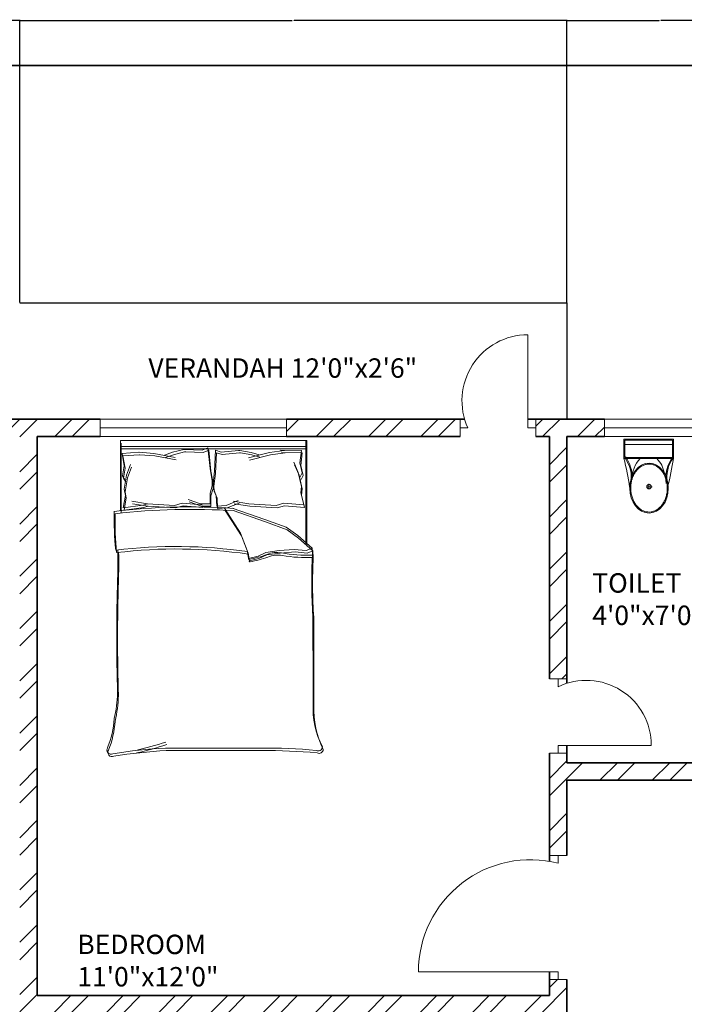
# Model space of a CAD drawing. Units: inches. Extents: x 1885 to 2748, y 783 to 2421.
# Tile 89 of 117: x 2170 to 2341, y 2167 to 2421. Entities that reach past the tile are written whole.
import ezdxf

# ---------------------------------------------------------------- set-up
doc = ezdxf.new("R2010")
doc.units = ezdxf.units.IN
for name, color, linetype, lineweight in [('A-ANNO-DIMS', 2, 'Continuous', 18), ('A-ANNO-TTLB', 7, 'Continuous', 35), ('A-AREA-IDEN', 7, 'Continuous', 18), ('A-DOOR', 31, 'Continuous', 18), ('A-FLOR-BALC', 7, 'Continuous', 25), ('A-FLOR-FIXT', 8, 'Continuous', 18), ('A-FURN', 8, 'Continuous', 13), ('A-GLAZ', 181, 'Continuous', 18), ('A-WALL', 7, 'Continuous', 35)]:
    doc.layers.add(name, color=color, linetype=linetype, lineweight=lineweight)
doc.layers.add('A-WALL-PATT', color=85, linetype='Continuous', lineweight=13, true_color=0x58ba48)
doc.styles.get("Standard").update_dxf_attribs({"font": 'arial.ttf'})
doc.dimstyles.get("Standard").update_dxf_attribs({"dimtxt": 0.18, "dimasz": 0.18, "dimexe": 0.18, "dimexo": 0.0625, "dimgap": 0.09, "dimtad": 0, "dimtih": 1, "dimtoh": 1, "dimdec": 4, "dimzin": 0, "dimdsep": 46, "dimtxsty": 'Standard', "dimcen": 0.09, "dimadec": 0, "dimazin": 0, "dimtfac": 1, "dimtdec": 4, "dimtofl": 0, "dimtmove": 0, "dimatfit": 3, "dimfxl": 1, "dimtolj": 1, "dimtzin": 0, "dimarcsym": 0})

# ---------------------------------------------------------------- blocks, each defined once
blk = doc.blocks.new('A$C31115884')
for p, q in [((258, 466), (258, 523)), ((283, 498), (223, 498)), ((0, 200), (0, 0)), ((520, 200), (0, 200)), ((10, 190), (10, 10)), ((510, 190), (10, 190)), ((510, 10), (510, 190)), ((520, 0), (520, 200)), ((510, 54), (0, 54)), ((10, 10), (510, 10)), ((0, 0), (520, 0))]:
    blk.add_line(p, q)
blk.add_circle((256, 496), 23.6)
for centre, radius, start, end in [((2778, -205), 2807, 165.4549, 171.7133), ((-295, 403), 365, 324.2091, 9.3499), ((-295, 403), 375, 324.2091, 9.3499), ((139, 406), 293, 315.8436, 2.6563), ((806, 403), 365, 170.6501, 215.7909), ((3237, 905), 2807, 188.2867, 194.5451), ((384, 406), 293, 190.2774, 224.1564), ((806, 403), 375, 179.2036, 215.7909)]:
    blk.add_arc(centre, radius, start, end)
blk.add_ellipse((256, 510), major_axis=(0, -261), ratio=0.772727)
blk.add_open_spline([(256, 259), (263, 259), (270, 260), (288, 262), (299, 265), (320, 273), (330, 278), (350, 291), (360, 299), (378, 316), (386, 326), (402, 347), (409, 358), (421, 383), (427, 395), (436, 422), (440, 436), (445, 465), (447, 480), (448, 509), (448, 524), (445, 553), (443, 568), (436, 596), (432, 610), (422, 636), (416, 649), (402, 672), (395, 683), (379, 703), (370, 712), (351, 728), (341, 735), (321, 746), (310, 751), (289, 757), (278, 759), (256, 761), (245, 761), (223, 757), (212, 754), (191, 746), (181, 741), (161, 728), (151, 720), (133, 703), (125, 693), (110, 672), (103, 660), (90, 636), (85, 623), (76, 596), (72, 582), (67, 553), (66, 538), (64, 509), (65, 494), (68, 465), (70, 450), (77, 422), (81, 408), (91, 382), (97, 370), (111, 346), (118, 335), (135, 316), (144, 307), (162, 291), (172, 284), (193, 273), (203, 269), (225, 262), (236, 260), (250, 259), (253, 259), (256, 259)], degree=3, knots=[0, 0, 0, 0, 0.110105, 0.110105, 0.285049, 0.285049, 0.459994, 0.459994, 0.634938, 0.634938, 0.809882, 0.809882, 0.984827, 0.984827, 1.159771, 1.159771, 1.334715, 1.334715, 1.50966, 1.50966, 1.684604, 1.684604, 1.859549, 1.859549, 2.034493, 2.034493, 2.209437, 2.209437, 2.384382, 2.384382, 2.559326, 2.559326, 2.73427, 2.73427, 2.909215, 2.909215, 3.084159, 3.084159, 3.259103, 3.259103, 3.434048, 3.434048, 3.608992, 3.608992, 3.783936, 3.783936, 3.958881, 3.958881, 4.133825, 4.133825, 4.30877, 4.30877, 4.483714, 4.483714, 4.658658, 4.658658, 4.833603, 4.833603, 5.008547, 5.008547, 5.183491, 5.183491, 5.358436, 5.358436, 5.53338, 5.53338, 5.708324, 5.708324, 5.883269, 5.883269, 6.058213, 6.058213, 6.233158, 6.233158, 6.283185, 6.283185, 6.283185, 6.283185])
blk = doc.blocks.new('BED-DOUBLE')
for p, q in [((0, 51.49), (0.64, 51.49)), ((0, 3.47), (0, 51.49)), ((0, 51.26), (26.61, 51.26)), ((0, 51.26), (26.61, 51.26)), ((0.64, 51.49), (27.25, 51.49)), ((0.64, 51.49), (27.25, 51.49)), ((1.54, 3.47), (1.54, 51.26)), ((1.54, 3.47), (1.54, 51.26)), ((2.18, 3.7), (2.18, 51.49)), ((2.18, 3.7), (2.18, 51.49)), ((17.22, 50.93), (14.08, 50.15)), ((17.22, 50.93), (14.08, 50.15)), ((16.81, 45.79), (17.22, 50.93)), ((16.81, 45.79), (17.22, 50.93)), ((27.75, 52.87), (24.5, 49.16)), ((27.75, 52.87), (24.5, 49.16)), ((28.39, 53.09), (25.14, 49.39)), ((28.39, 53.09), (25.14, 49.39)), ((29.49, 52.95), (27.75, 52.87, 3.87)), ((29.49, 52.95), (27.75, 52.87, 3.87)), ((28.37, 51.33), (27.75, 52.87)), ((28.37, 51.33), (27.75, 52.87)), ((28.06, 48.23), (28.37, 51.33)), ((28.06, 48.23), (28.37, 51.33)), ((30.13, 53.17), (28.39, 53.09, 3.87)), ((30.13, 53.17), (28.39, 53.09, 3.87)), ((29.01, 51.56), (28.39, 53.09)), ((29.01, 51.56), (28.39, 53.09)), ((28.7, 48.46), (29.01, 51.56)), ((28.7, 48.46), (29.01, 51.56)), ((2.56, 50.11), (2.46, 44.71)), ((2.56, 50.11), (2.46, 44.71)), ((2.56, 50.11), (5.77, 49.73)), ((2.56, 50.11), (5.77, 49.73)), ((3.2, 50.34), (3.1, 44.94)), ((3.2, 50.34), (3.1, 44.94)), ((3.2, 50.34), (6.41, 49.96)), ((3.2, 50.34), (6.41, 49.96)), ((8.26, 49.31), (5.58, 48.13)), ((8.26, 49.31), (5.58, 48.13)), ((5.77, 49.73), (8.34, 50.33)), ((5.77, 49.73), (8.34, 50.33)), ((8.9, 49.54), (6.22, 48.36)), ((8.9, 49.54), (6.22, 48.36)), ((6.41, 49.96), (8.98, 50.56)), ((6.41, 49.96), (8.98, 50.56)), ((11.83, 50.11), (8.26, 49.31)), ((11.83, 50.11), (8.26, 49.31)), ((8.34, 50.33), (9.39, 49.81)), ((8.34, 50.33), (9.39, 49.81)), ((12.47, 50.34), (8.9, 49.54)), ((12.47, 50.34), (8.9, 49.54)), ((8.98, 50.56), (10.03, 50.04)), ((8.98, 50.56), (10.03, 50.04)), ((13.44, 49.92), (11.83, 50.11)), ((13.44, 49.92), (11.83, 50.11)), ((14.08, 50.15), (12.47, 50.34)), ((14.08, 50.15), (12.47, 50.34)), ((16.58, 50.7), (13.44, 49.92)), ((16.58, 50.7), (13.44, 49.92)), ((16.17, 45.57), (16.58, 50.7)), ((16.17, 45.56), (16.58, 50.7)), ((24.5, 49.16), (22.33, 46.22)), ((24.5, 49.16), (22.33, 46.22)), ((25.14, 49.39), (22.97, 46.45)), ((25.14, 49.39), (22.97, 46.45)), ((28.37, 44.36), (28.06, 48.23)), ((28.37, 44.36), (28.06, 48.23)), ((29.01, 44.59), (28.7, 48.46)), ((29.01, 44.59), (28.7, 48.46)), ((2.46, 44.71), (2.55, 45.71)), ((2.46, 44.71), (2.55, 45.71)), ((2.55, 45.71), (3.07, 41.91)), ((2.55, 45.71), (3.07, 41.91)), ((3.1, 44.94), (3.19, 45.94)), ((3.1, 44.94), (3.19, 45.94)), ((3.19, 45.94), (3.71, 42.14)), ((3.19, 45.94), (3.71, 42.14)), ((17.37, 43.83), (16.81, 45.79)), ((17.37, 43.83), (16.81, 45.79)), ((22.33, 46.22), (20.32, 40.64)), ((22.33, 46.22), (20.32, 40.64)), ((22.97, 46.45), (20.96, 40.87)), ((22.97, 46.45), (20.96, 40.87)), ((16.73, 43.6), (16.17, 45.57)), ((16.73, 43.6), (16.17, 45.56)), ((16.3, 36.59), (16.73, 43.6)), ((16.3, 36.59), (16.73, 43.6)), ((16.94, 36.82), (17.37, 43.83)), ((16.94, 36.82), (17.37, 43.83)), ((28.83, 40.95), (28.37, 44.36)), ((28.83, 40.95), (28.37, 44.36)), ((29.47, 41.18), (29.01, 44.59)), ((29.47, 41.18), (29.01, 44.59)), ((3.07, 41.91), (4.43, 36.49)), ((3.07, 41.91), (4.43, 36.49)), ((3.71, 42.14), (5.07, 36.72)), ((3.71, 42.14), (5.07, 36.72)), ((20.32, 40.64), (17.39, 32.3)), ((20.32, 40.64), (17.39, 32.3)), ((20.96, 40.87), (18.03, 32.53)), ((20.96, 40.87), (18.03, 32.53)), ((29.76, 38.94), (28.83, 40.95)), ((29.76, 38.94), (28.83, 40.95)), ((30.4, 39.17), (29.47, 41.18)), ((30.4, 39.17), (29.47, 41.18)), ((3.68, 39.2), (3.08, 37.13)), ((3.68, 39.2), (3.08, 37.13)), ((4.32, 39.43), (3.72, 37.36)), ((4.32, 39.43), (3.72, 37.36)), ((30.38, 36.46), (29.76, 38.94)), ((30.38, 36.46), (29.76, 38.94)), ((31.02, 36.69), (30.4, 39.17)), ((31.02, 36.69), (30.4, 39.17)), ((79.25, 15.06), (79.25, 39.68)), ((79.25, 15.06), (79.25, 39.68)), ((79.89, 15.29), (79.89, 39.9)), ((79.89, 15.29), (79.89, 39.9)), ((3.08, 37.13), (2.54, 34.2)), ((3.08, 37.13), (2.54, 34.2)), ((3.72, 37.36), (3.18, 34.43)), ((3.72, 37.36), (3.18, 34.43)), ((15.63, 32.56), (16.3, 36.59)), ((15.63, 32.56), (16.3, 36.59)), ((16.27, 32.79), (16.94, 36.82)), ((16.27, 32.79), (16.94, 36.82)), ((23.88, 34.45), (28.37, 36.15)), ((23.88, 34.45), (28.37, 36.15)), ((24.52, 34.68), (29.01, 36.38)), ((24.52, 34.68), (29.01, 36.38)), ((28.37, 36.15), (30.38, 36.46)), ((28.37, 36.15), (30.38, 36.46)), ((29.01, 36.38), (31.02, 36.69)), ((29.01, 36.38), (31.02, 36.69)), ((2.54, 34.2), (2.56, 33.88)), ((2.54, 34.2), (2.56, 33.88)), ((2.56, 33.88), (2.98, 29.45)), ((2.56, 33.88), (2.98, 29.45)), ((3.18, 34.43), (3.2, 34.11)), ((3.18, 34.43), (3.2, 34.11)), ((3.2, 34.11), (3.62, 29.68)), ((3.2, 34.11), (3.62, 29.68)), ((16.74, 30.75), (15.46, 33.82)), ((16.74, 30.75), (15.46, 33.82)), ((17.38, 30.98), (16.1, 34.05)), ((17.38, 30.98), (16.1, 34.05)), ((17.39, 30.26), (23.88, 34.45)), ((17.39, 30.26), (23.88, 34.45)), ((18.03, 30.49), (24.52, 34.68)), ((18.03, 30.49), (24.52, 34.68)), ((16.9, 28.3), (16.74, 30.75)), ((16.9, 28.3), (16.74, 30.75)), ((17.54, 28.52), (17.38, 30.98)), ((17.54, 28.52), (17.38, 30.98)), ((2.98, 29.45), (2.5, 27.98)), ((2.98, 29.45), (2.5, 27.98)), ((2.5, 27.98), (7.87, 27.73)), ((2.5, 27.98), (7.87, 27.73)), ((3.62, 29.68), (3.13, 28.2)), ((3.62, 29.68), (3.13, 28.2)), ((3.13, 28.2), (8.51, 27.96)), ((3.13, 28.2), (8.51, 27.96)), ((8.51, 27.96), (11.72, 27.58)), ((8.51, 27.96), (11.72, 27.58)), ((12.38, 27.43), (14.22, 28.13)), ((12.38, 27.43), (14.22, 28.13)), ((13.02, 27.66), (14.86, 28.36)), ((13.02, 27.66), (14.86, 28.36)), ((14.22, 28.13), (16.9, 28.3)), ((14.22, 28.13), (16.9, 28.3)), ((14.86, 28.36), (17.54, 28.52)), ((14.86, 28.36), (17.54, 28.52)), ((1.87, 25.98), (7.22, 26.56)), ((1.87, 25.98), (7.22, 26.56)), ((2.45, 24.54), (1.87, 25.98)), ((2.45, 24.54), (1.87, 25.98)), ((2.51, 26.21), (7.86, 26.79)), ((2.51, 26.21), (7.86, 26.79)), ((3.09, 24.76), (2.51, 26.21)), ((3.09, 24.76), (2.51, 26.21)), ((7.22, 26.56), (10.4, 27.14)), ((7.22, 26.56), (10.4, 27.14)), ((7.86, 26.79), (11.04, 27.37)), ((7.86, 26.79), (11.04, 27.37)), ((7.87, 27.73), (11.08, 27.35)), ((7.87, 27.73), (11.08, 27.35)), ((10.4, 27.14), (11.71, 27.14)), ((10.4, 27.14), (11.71, 27.14)), ((11.04, 27.37), (12.35, 27.37)), ((11.04, 27.37), (12.35, 27.37)), ((11.08, 27.35), (12.38, 27.43)), ((11.08, 27.35), (12.38, 27.43)), ((11.71, 27.14), (13.59, 26.56)), ((11.71, 27.14), (13.59, 26.56)), ((11.72, 27.58), (13.02, 27.66)), ((11.72, 27.58), (13.02, 27.66)), ((12.35, 27.37), (14.22, 26.79)), ((12.35, 27.37), (14.22, 26.79)), ((13.59, 26.56), (16.27, 26.56)), ((13.59, 26.56), (16.27, 26.56)), ((14.22, 26.79), (16.91, 26.79)), ((14.22, 26.79), (16.91, 26.79)), ((16.27, 26.56), (16.27, 24.1)), ((16.27, 26.56), (16.27, 24.1)), ((16.91, 26.79), (16.91, 24.33)), ((16.91, 26.79), (16.91, 24.33)), ((2.31, 20.09), (2.45, 24.54)), ((2.31, 20.09), (2.45, 24.54)), ((2.95, 20.32), (3.09, 24.76)), ((2.95, 20.32), (3.09, 24.76)), ((16.27, 24.1), (15.18, 20.96)), ((16.27, 24.1), (15.18, 20.96)), ((16.91, 24.33), (15.82, 21.19)), ((16.91, 24.33), (15.82, 21.19)), ((16.17, 19.38), (16.58, 24.51)), ((16.17, 19.38), (16.58, 24.51)), ((16.81, 19.61), (17.22, 24.74)), ((16.81, 19.61), (17.22, 24.74)), ((2.95, 20), (2.95, 20.32)), ((2.95, 20), (2.95, 20.32)), ((2.31, 19.77), (2.31, 20.09)), ((2.31, 19.77), (2.31, 20.09)), ((3.03, 16.88), (2.31, 19.77)), ((3.03, 16.88), (2.31, 19.77)), ((3.67, 17.11), (2.95, 20)), ((3.67, 17.11), (2.95, 20)), ((3.96, 12.34), (4.97, 17.83)), ((3.96, 12.34), (4.97, 17.83)), ((16.73, 17.42), (16.17, 19.38)), ((16.73, 17.42), (16.17, 19.38)), ((17.37, 17.65), (16.81, 19.61)), ((17.37, 17.65), (16.81, 19.61)), ((3.75, 14.85), (3.03, 16.88)), ((3.75, 14.85), (3.03, 16.88)), ((3.32, 12.11), (4.33, 17.6)), ((3.32, 12.11), (4.33, 17.6)), ((4.39, 15.08), (3.67, 17.11)), ((4.39, 15.08), (3.67, 17.11)), ((16.3, 10.41), (16.73, 17.42)), ((16.3, 10.41), (16.73, 17.42)), ((16.94, 10.64), (17.37, 17.65)), ((16.94, 10.64), (17.37, 17.65)), ((3.03, 8.28), (3.32, 12.11)), ((3.03, 8.28), (3.32, 12.11)), ((3.67, 8.51), (3.96, 12.34)), ((3.67, 8.51), (3.96, 12.34)), ((15.63, 6.38), (16.3, 10.41)), ((15.63, 6.38), (16.3, 10.41)), ((16.27, 6.61), (16.94, 10.64)), ((16.27, 6.61), (16.94, 10.64)), ((16.3, 10.41), (16.62, 9.28)), ((16.3, 10.41), (16.62, 9.28)), ((16.94, 10.64), (17.26, 9.51)), ((16.94, 10.64), (17.26, 9.51)), ((3.01, 8.18), (3.03, 8.28)), ((3.01, 8.18), (3.03, 8.28)), ((3.34, 3.9), (3.01, 8.18)), ((3.34, 3.9), (3.01, 8.18)), ((3.65, 8.41), (3.67, 8.51)), ((3.65, 8.41), (3.67, 8.51)), ((3.98, 4.13), (3.65, 8.41)), ((3.98, 4.13), (3.65, 8.41)), ((16.62, 9.28), (17.34, 4.18)), ((16.62, 9.28), (17.34, 4.18)), ((17.26, 9.51), (17.98, 4.41)), ((17.26, 9.51), (17.98, 4.41)), ((8.96, 5.05), (6.21, 6.06)), ((8.96, 5.05), (6.21, 6.06)), ((9.6, 5.28), (6.85, 6.29)), ((9.6, 5.28), (6.85, 6.29)), ((13.21, 4.7), (9.6, 5.28)), ((13.21, 4.7), (9.6, 5.28)), ((18.11, 3.47), (0, 3.47)), ((18.11, 3.47), (0, 3.47)), ((18.75, 3.7), (0.64, 3.7)), ((18.75, 3.7), (0.64, 3.7)), ((3.32, 3.89), (6.5, 4.47)), ((3.32, 3.89), (6.5, 4.47)), ((3.96, 4.12), (7.14, 4.7)), ((3.96, 4.12), (7.14, 4.7)), ((6.5, 4.47), (9.1, 4.04)), ((6.5, 4.47), (9.1, 4.04)), ((7.14, 4.7), (9.74, 4.27)), ((7.14, 4.7), (9.74, 4.27)), ((12.57, 4.47), (8.96, 5.05)), ((12.57, 4.47), (8.96, 5.05)), ((9.1, 4.04), (10.12, 4.62)), ((9.1, 4.04), (10.12, 4.62)), ((9.74, 4.27), (10.75, 4.84)), ((9.74, 4.27), (10.75, 4.84)), ((14.16, 4.76), (12.57, 4.47)), ((14.16, 4.76), (12.57, 4.47)), ((14.8, 4.99), (13.21, 4.7)), ((14.8, 4.99), (13.21, 4.7)), ((17.34, 4.18), (14.16, 4.76)), ((17.34, 4.18), (14.16, 4.76)), ((17.98, 4.41), (14.8, 4.99)), ((17.98, 4.41), (14.8, 4.99))]:
    blk.add_line(p, q)
for centre, radius, start, end in [((36.96, 182.49), 129.5, 266.9791, 273.8365), ((36.96, 182.49), 129.5, 266.9791, 273.8365), ((68.46, -4508.52), 4561.86, 90.00217, 90.28689), ((68.46, -4508.52), 4561.86, 90.00217, 90.28689), ((68.67, 76.16), 23.07, 267.4714, 296.4681), ((68.67, 76.16), 23.07, 267.4714, 296.4681), ((69.31, 76.38), 23.07, 267.4714, 296.4681), ((69.31, 76.38), 23.07, 267.4714, 296.4681), ((78.87, 54.41), 1.1, 332.6588, 86.02), ((78.87, 54.41), 1.1, 332.6588, 86.02), ((212.28, 41.15), 133.04, 174.4998, 180.6351), ((212.28, 41.15), 133.04, 174.4998, 180.6351), ((79.51, 54.64), 1.1, 332.6588, 86.02), ((79.51, 54.64), 1.1, 332.6588, 86.02), ((212.92, 41.38), 133.04, 174.4998, 180.6351), ((212.92, 41.38), 133.04, 174.4998, 180.6351), ((-6.65, 51.33), 36.18, 349.8763, 2.5657), ((-6.65, 51.33), 36.18, 349.8763, 2.5657), ((36.32, 182.26), 129.5, 266.9791, 273.8365), ((36.32, 182.26), 129.5, 266.9791, 273.8365), ((-6.01, 51.55), 36.18, 349.8763, 2.5657), ((-6.01, 51.55), 36.18, 349.8763, 2.5657), ((67.83, -4508.74), 4561.86, 90.00217, 90.28689), ((67.83, -4508.75), 4561.86, 90.00217, 90.28689), ((35.07, 43.74), 6.22, 168.6608, 203.7384), ((35.07, 43.74), 6.22, 168.6608, 203.7384), ((35.71, 43.97), 6.22, 168.6608, 203.7384), ((35.71, 43.97), 6.22, 168.6608, 203.7384), ((1.49, 31.15), 29.65, 10.6617, 19.8806), ((1.49, 31.15), 29.65, 10.6617, 19.8806), ((2.13, 31.38), 29.65, 10.6617, 19.8806), ((2.13, 31.38), 29.65, 10.6617, 19.8806), ((156.32, 17.75), 129.02, 171.7845, 186.9006), ((156.32, 17.75), 129.02, 171.7845, 186.9006), ((156.96, 17.98), 129.02, 171.7845, 186.9006), ((156.96, 17.98), 129.02, 171.7845, 186.9006), ((30.44, 36.64), 0.185, 250.2464, 1.1377), ((30.44, 36.63), 0.185, 250.2464, 1.1377), ((31.08, 36.86), 0.185, 250.2464, 1.1377), ((31.08, 36.86), 0.185, 250.2464, 1.1377), ((182.06, 21.36), 164.97, 176.0865, 186.7821), ((182.06, 21.36), 164.97, 176.0865, 186.7821), ((182.7, 21.59), 164.97, 176.0865, 186.7821), ((182.7, 21.59), 164.97, 176.0865, 186.7821), ((-23.07, -16.99), 106.46, 13.3832, 17.7053), ((-23.07, -16.99), 106.46, 13.3832, 17.7053), ((201.48, 21.65), 121.76, 182.9958, 189.4091), ((201.48, 21.65), 121.76, 182.9958, 189.4091), ((-23.71, -17.22), 106.46, 13.3832, 17.7053), ((-23.71, -17.22), 106.46, 13.3832, 17.7053), ((200.84, 21.43), 121.76, 182.9958, 189.4091), ((200.84, 21.43), 121.76, 182.9958, 189.4091), ((31.18, -167.31), 170.11, 88.4762, 91.0082), ((31.18, -167.31), 170.11, 88.4762, 91.0082), ((31.82, -167.08), 170.11, 88.4762, 91.0082), ((31.82, -167.08), 170.11, 88.4762, 91.0082), ((50.62, 484.82), 482.31, 268.2277, 271.7185), ((50.62, 484.82), 482.31, 268.2277, 271.7185), ((51.26, 485.05), 482.31, 268.2277, 271.7185), ((51.26, 485.05), 482.31, 268.2277, 271.7185), ((64.52, -26.9), 29.63, 76.0648, 88.9113), ((64.52, -26.9), 29.63, 76.0648, 88.9113), ((65.16, -26.67), 29.63, 76.0648, 88.9113), ((65.16, -26.67), 29.63, 76.0648, 88.9113), ((20.1, 85.16), 83.31, 268.7218, 275.604), ((20.1, 85.16), 83.31, 268.7218, 275.604), ((20.74, 85.39), 83.31, 268.7218, 275.604), ((20.74, 85.39), 83.31, 268.7218, 275.604), ((70.28, -21.66), 23.56, 67.9751, 86.652), ((70.28, -21.66), 23.56, 67.9751, 86.652), ((70.92, -21.43), 23.56, 67.9751, 86.652), ((70.92, -21.43), 23.56, 67.9751, 86.652), ((79.72, 1.09), 1.09, 236.1736, 23.4781), ((79.72, 1.09), 1.09, 236.1736, 23.4781), ((80.36, 1.31), 1.09, 236.1736, 23.4781), ((80.36, 1.31), 1.09, 236.1736, 23.4781)]:
    blk.add_arc(centre, radius, start, end)
blk = doc.blocks.new('WIN-24')
for p, q in [((0, 4.5), (0, 0)), ((0, 4.5), (24, 4.5)), ((24, 2.25), (24, 4.5)), ((24, 4.5), (24, 0)), ((0, 0), (0, 2.25)), ((0, 2.25), (24, 2.25)), ((24, 0), (0, 0))]:
    blk.add_line(p, q)
blk = doc.blocks.new('WIN-48')
for p, q in [((0, 4.5), (0, 0)), ((48, 4.5), (0, 4.5)), ((48, 2.25), (48, 4.5)), ((48, 4.5), (48, 0)), ((0, 0), (0, 2.25)), ((0, 2.25), (48, 2.25)), ((0, 0), (48, 0))]:
    blk.add_line(p, q)
blk = doc.blocks.new('*D50')
at = {"layer": 'A-ANNO-DIMS', "color": 0, "lineweight": -2, "transparency": 16777216}
for p, q in [((2121.77, 2348.07), (2121.77, 2420.94)), ((2121.95, 2420.76), (2145.55, 2420.76)), ((2169.59, 2420.76), (2146, 2420.76)), ((2169.77, 2348.07), (2169.77, 2420.94))]:
    blk.add_line(p, q, dxfattribs=at)
at = {"layer": 'A-ANNO-DIMS', "color": 0, "transparency": 16777216}
for points in [[(2121.95, 2420.79), (2121.95, 2420.73), (2121.77, 2420.76)], [(2169.59, 2420.79), (2169.59, 2420.73), (2169.77, 2420.76)]]:
    blk.add_solid(points, dxfattribs=at)
at = {"layer": 'Defpoints', "color": 0, "transparency": 16777216}
for p in [(2169.77, 2420.76), (2121.77, 2348.01), (2169.77, 2348.01)]:
    blk.add_point(p, dxfattribs=at)
at = {"layer": 'A-ANNO-DIMS', "color": 0, "transparency": 16777216, "insert": (2145.77, 2420.76), "char_height": 0.18, "attachment_point": 5}
blk.add_mtext('\\A1;48', dxfattribs=at)
blk = doc.blocks.new('*D51')
at = {"layer": 'A-ANNO-DIMS', "color": 0, "lineweight": -2, "transparency": 16777216}
for p, q in [((2169.77, 2348.07), (2169.77, 2420.94)), ((2169.95, 2420.76), (2240.01, 2420.76)), ((2310.59, 2420.76), (2240.54, 2420.76)), ((2310.77, 2348.07), (2310.77, 2420.94))]:
    blk.add_line(p, q, dxfattribs=at)
at = {"layer": 'A-ANNO-DIMS', "color": 0, "transparency": 16777216}
for points in [[(2169.95, 2420.79), (2169.95, 2420.73), (2169.77, 2420.76)], [(2310.59, 2420.79), (2310.59, 2420.73), (2310.77, 2420.76)]]:
    blk.add_solid(points, dxfattribs=at)
at = {"layer": 'Defpoints', "color": 0, "transparency": 16777216}
for p in [(2310.77, 2420.76), (2169.77, 2348.01), (2310.77, 2348.01)]:
    blk.add_point(p, dxfattribs=at)
at = {"layer": 'A-ANNO-DIMS', "color": 0, "transparency": 16777216, "insert": (2240.27, 2420.76), "char_height": 0.18, "attachment_point": 5}
blk.add_mtext('\\A1;141', dxfattribs=at)
blk = doc.blocks.new('*D52')
at = {"layer": 'A-ANNO-DIMS', "color": 0, "lineweight": -2, "transparency": 16777216}
for p, q in [((2310.77, 2348.07), (2310.77, 2420.94)), ((2310.95, 2420.76), (2334.55, 2420.76)), ((2358.59, 2420.76), (2335, 2420.76)), ((2358.77, 2352.57), (2358.77, 2420.94))]:
    blk.add_line(p, q, dxfattribs=at)
at = {"layer": 'A-ANNO-DIMS', "color": 0, "transparency": 16777216}
for points in [[(2310.95, 2420.79), (2310.95, 2420.73), (2310.77, 2420.76)], [(2358.59, 2420.79), (2358.59, 2420.73), (2358.77, 2420.76)]]:
    blk.add_solid(points, dxfattribs=at)
at = {"layer": 'Defpoints', "color": 0, "transparency": 16777216}
for p in [(2358.77, 2420.76), (2358.77, 2352.51), (2310.77, 2348.01)]:
    blk.add_point(p, dxfattribs=at)
at = {"layer": 'A-ANNO-DIMS', "color": 0, "transparency": 16777216, "insert": (2334.77, 2420.76), "char_height": 0.18, "attachment_point": 5}
blk.add_mtext('\\A1;48', dxfattribs=at)

msp = doc.modelspace()

# ---------------------------------------------------------------- hatches: boundary and pattern name
at = {"layer": 'A-WALL-PATT'}
h = msp.add_hatch(dxfattribs=at)
h.set_pattern_fill('ANSI32', color=256)
h.paths.add_polyline_path([(2007.77, 2318.01), (1980.77, 2318.01), (1980.77, 2281.22), (1985.27, 2281.22), (1985.27, 2313.51), (2007.77, 2313.51), (2007.77, 2315.76)])
h.paths.add_polyline_path([(2094.32, 2318.01), (2067.77, 2318.01), (2067.77, 2313.51), (2094.32, 2313.51), (2094.32, 2315.76)])
h.paths.add_polyline_path([(2131.37, 2315.76), (2131.37, 2318.01), (2131.19, 2318.01), (2112.61, 2318.01), (2112.61, 2313.51), (2117.27, 2313.51), (2117.27, 2255.2), (2121.77, 2255.2), (2121.77, 2313.51), (2131.37, 2313.51)])
h.paths.add_polyline_path([(2190.51, 2318.01), (2155.37, 2318.01), (2155.37, 2313.51), (2169.77, 2313.51), (2169.77, 2229.51), (2121.77, 2229.51), (2121.77, 2233.45), (2119.52, 2233.45), (2117.27, 2233.45), (2117.27, 2201.1), (2121.77, 2201.1), (2121.77, 2225.01), (2169.77, 2225.01), (2169.77, 2165.01), (2306.27, 2165.01), (2306.27, 2066.01), (2310.77, 2066.01), (2344.27, 2066.01), (2486.27, 2066.01), (2486.27, 1886.01), (2483.02, 1886.01), (2483.02, 1881.51), (2486.27, 1881.51), (2486.27, 1880.68), (2490.77, 1880.68), (2490.77, 2070.51), (2344.27, 2070.51), (2310.77, 2070.51), (2310.77, 2165.01), (2310.77, 2173.64), (2308.52, 2173.64), (2306.27, 2173.64), (2306.27, 2169.51), (2174.27, 2169.51), (2174.27, 2313.51), (2190.51, 2313.51), (2190.51, 2315.76)])
h.paths.add_polyline_path([(1985.27, 2221.22), (1980.77, 2221.22), (1980.77, 2165.01), (1992.77, 2165.01), (1992.77, 2141.93), (1997.27, 2141.93), (1997.27, 2165.01), (2117.27, 2165.01), (2117.27, 2163.13), (2121.77, 2163.13), (2121.77, 2172.73), (2119.52, 2172.73), (2117.27, 2172.73), (2117.27, 2169.51), (1985.27, 2169.51)])
h.paths.add_polyline_path([(1997.27, 2105.93), (1992.77, 2105.93), (1992.77, 2070.51), (2016.77, 2070.51), (2016.77, 2059.12), (2019.02, 2059.12), (2021.27, 2059.12), (2021.27, 2070.51), (2117.27, 2070.51), (2117.27, 2022.51), (2114.42, 2022.51), (2114.42, 2018.01), (2123.63, 2018.01), (2123.63, 2020.26), (2123.63, 2022.51), (2121.77, 2022.51), (2121.77, 2142.59), (2119.52, 2142.59), (2117.27, 2142.59), (2117.27, 2075.01), (1997.27, 2075.01)])
h.paths.add_polyline_path([(2092.03, 2020.26), (2092.03, 2022.51), (2021.27, 2022.51), (2021.27, 2035.12), (2016.77, 2035.12), (2016.77, 2018.01), (2016.77, 1978.78), (2021.27, 1978.78), (2021.27, 2018.01), (2092.03, 2018.01)])
h.paths.add_polyline_path([(2260.94, 2022.51), (2153.1, 2022.51), (2153.1, 2020.26), (2153.1, 2018.01), (2155.27, 2018.01), (2155.27, 1886.01), (2107.63, 1886.01), (2107.63, 1881.51), (2182.91, 1881.51), (2182.91, 1883.76), (2182.91, 1886.01), (2159.77, 1886.01), (2159.77, 2018.01), (2260.94, 2018.01), (2260.94, 2020.26)])
h.paths.add_polyline_path([(2047.63, 1883.76), (2047.63, 1886.01), (2021.27, 1886.01), (2021.27, 1918.78), (2019.02, 1918.78), (2016.77, 1918.78), (2016.77, 1881.51), (2047.63, 1881.51)])
h.paths.add_polyline_path([(2306.36, 1883.76), (2306.36, 1886.01), (2296.27, 1886.01), (2296.27, 1982.01), (2316.54, 1982.01), (2316.54, 1984.26), (2316.54, 1986.51), (2296.27, 1986.51), (2296.27, 2022.51), (2289.28, 2022.51), (2289.28, 2018.01), (2291.77, 2018.01), (2291.77, 1886.01), (2242.91, 1886.01), (2242.91, 1881.51), (2306.36, 1881.51)], flags=17)
h.paths.add_polyline_path([(1985.27, 1843.01), (2021.6, 1843.01), (2021.53, 1845.44), (2021.48, 1847.51), (1980.77, 1847.51), (1980.77, 1809.45), (1985.27, 1809.45)])
h.paths.add_polyline_path([(2131.48, 1845.26), (2131.48, 1847.51), (2081.53, 1847.51), (2081.53, 1843.01), (2117.27, 1843.01), (2117.27, 1784.15), (2119.52, 1784.15), (2121.77, 1784.15), (2121.77, 1843.01), (2131.48, 1843.01)])
h.paths.add_polyline_path([(2203.89, 1847.51), (2155.48, 1847.51), (2155.48, 1843.01), (2169.77, 1843.01), (2169.77, 1759.01), (2121.77, 1759.01), (2121.77, 1761.46), (2117.27, 1761.46), (2117.27, 1730.43), (2121.77, 1730.43), (2121.77, 1754.51), (2177.42, 1754.51), (2177.42, 1756.76), (2177.42, 1759.01), (2174.27, 1759.01), (2174.27, 1843.01), (2203.89, 1843.01)])
h.paths.add_polyline_path([(2335.55, 1845.26), (2335.55, 1847.51), (2239.89, 1847.51), (2239.89, 1843.01), (2306.27, 1843.01), (2306.27, 1759.01), (2199.49, 1759.01), (2199.49, 1754.51), (2310.77, 1754.51), (2310.77, 1843.01), (2335.55, 1843.01)])
h.paths.add_polyline_path([(2348.77, 2022.51), (2344.27, 2022.51), (2344.27, 1986.51), (2341.68, 1986.51), (2341.68, 1982.01), (2344.27, 1982.01), (2344.27, 1886.01), (2330.36, 1886.01), (2330.36, 1881.51), (2361.63, 1881.51), (2361.63, 1883.76), (2361.63, 1886.01), (2348.77, 1886.01)], flags=17)
h.paths.add_polyline_path([(2283.25, 2315.76), (2283.25, 2318.01), (2238.51, 2318.01), (2238.51, 2313.51), (2283.25, 2313.51)], flags=17)
h.paths.add_polyline_path([(2363.27, 2348.01), (2388.68, 2348.01), (2388.68, 2350.26), (2388.68, 2352.51), (2358.77, 2352.51), (2358.77, 2348.01), (2358.77, 2318.01), (2344.48, 2318.01), (2344.48, 2313.51), (2358.77, 2313.51), (2358.77, 2229.51), (2310.77, 2229.51), (2310.77, 2231.95), (2306.27, 2231.95), (2306.27, 2205.61), (2310.77, 2205.61), (2310.77, 2225.01), (2358.77, 2225.01), (2358.77, 2211.51), (2452.33, 2211.51), (2452.33, 2213.76), (2452.33, 2216.01), (2363.27, 2216.01), (2363.27, 2318.01)])
h.paths.add_polyline_path([(2310.77, 2313.51), (2320.48, 2313.51), (2320.48, 2315.76), (2320.48, 2318.01), (2302.73, 2318.01), (2302.73, 2313.51), (2306.27, 2313.51), (2306.27, 2251.08), (2310.77, 2251.08)], flags=17)
h.paths.add_polyline_path([(2490.77, 2352.51), (2486.27, 2352.51), (2448.68, 2352.51), (2448.68, 2348.01), (2486.27, 2348.01), (2486.27, 2318.01), (2486.27, 2216.01), (2481.78, 2216.01), (2481.78, 2211.51), (2486.27, 2211.51), (2486.27, 2165.01), (2493.29, 2165.01), (2493.29, 2167.26), (2493.29, 2169.51), (2490.77, 2169.51), (2490.77, 2313.51), (2494.43, 2313.51), (2494.43, 2318.01), (2490.77, 2318.01)])
h.paths.add_polyline_path([(2534.65, 2318.01), (2515.69, 2318.01), (2515.69, 2313.51), (2534.65, 2313.51), (2534.65, 2315.76)])
h.paths.add_polyline_path([(2618.27, 2318.01), (2594.65, 2318.01), (2594.65, 2313.51), (2613.77, 2313.51), (2613.77, 2281.71), (2618.27, 2281.71)])
h.paths.add_polyline_path([(2618.27, 2221.71), (2613.77, 2221.71), (2613.77, 2169.51), (2554.02, 2169.51), (2554.02, 2165.01), (2613.77, 2165.01), (2613.77, 2152.88), (2618.27, 2152.88)])
h.paths.add_polyline_path([(2618.27, 2128.88), (2616.02, 2128.88), (2613.77, 2128.88), (2613.77, 2117.01), (2529.77, 2117.01), (2529.77, 2165.01), (2532.85, 2165.01), (2532.85, 2169.51), (2522.87, 2169.51), (2522.87, 2165.01), (2525.27, 2165.01), (2525.27, 2117.01), (2525.27, 2112.51), (2525.27, 2108.58), (2529.77, 2108.58), (2529.77, 2112.51), (2613.77, 2112.51), (2613.77, 2080.19), (2618.27, 2080.19)])
h.paths.add_polyline_path([(2618.27, 2044.19), (2616.02, 2044.19), (2613.77, 2044.19), (2613.77, 2015.51), (2529.77, 2015.51), (2529.77, 2088.58), (2527.52, 2088.58), (2525.27, 2088.58), (2525.27, 2011.01), (2613.77, 2011.01), (2613.77, 1956.75), (2618.27, 1956.75)])
h.paths.add_polyline_path([(2618.27, 1881.51), (2618.27, 1896.75), (2613.77, 1896.75), (2613.77, 1881.51), (2613.77, 1847.51), (2592.71, 1847.51), (2592.71, 1843.01), (2613.77, 1843.01), (2613.77, 1765.01), (2613.77, 1760.51), (2609.62, 1760.51), (2609.62, 1756.01), (2613.77, 1756.01), (2613.77, 1660.01), (2608.54, 1660.01), (2608.54, 1655.51), (2613.77, 1655.51), (2613.77, 1508.16), (2618.27, 1508.16)])
h.paths.add_polyline_path([(2565.77, 1843.01), (2569, 1843.01), (2569, 1847.51), (2490.77, 1847.51), (2490.77, 1849.7), (2488.52, 1849.7), (2486.27, 1849.7), (2486.27, 1847.51), (2477.27, 1847.51), (2477.27, 1838.51), (2477.27, 1821.49), (2486.27, 1821.49), (2486.27, 1838.51), (2561.27, 1838.51), (2561.27, 1765.01), (2486.27, 1765.01), (2486.27, 1786.16), (2477.27, 1786.16), (2477.27, 1765.01), (2477.27, 1756.01), (2486.27, 1756.01), (2565.77, 1756.01), (2585.62, 1756.01), (2585.62, 1758.26), (2585.62, 1760.51), (2565.77, 1760.51), (2565.77, 1765.01)])
h.paths.add_polyline_path([(2486.27, 1651.01), (2561.27, 1651.01), (2561.27, 1567.01), (2486.27, 1567.01), (2486.27, 1591.32), (2477.27, 1591.32), (2477.27, 1567.01), (2477.27, 1558.01), (2477.27, 1555.44), (2481.77, 1555.44), (2481.77, 1558.01), (2568.65, 1558.01), (2568.65, 1560.26), (2568.65, 1562.51), (2565.77, 1562.51), (2565.77, 1655.51), (2584.54, 1655.51), (2584.54, 1657.76), (2584.54, 1660.01), (2565.77, 1660.01), (2486.27, 1660.01), (2477.27, 1660.01), (2477.27, 1651.01), (2477.27, 1632.99), (2486.27, 1632.99)])
h.paths.add_polyline_path([(2449.97, 1883.76), (2449.97, 1886.01), (2421.63, 1886.01), (2421.63, 1881.51), (2449.97, 1881.51)], flags=17)
h.paths.add_polyline_path([(2447.27, 1847.51), (2395.55, 1847.51), (2395.55, 1843.01), (2442.77, 1843.01), (2442.77, 1809.27), (2447.27, 1809.27)])
h.paths.add_polyline_path([(1985.27, 1749.45), (1980.77, 1749.45), (1980.77, 1694.5), (1985.27, 1694.5), (1985.27, 1694.51), (1986.9, 1694.51), (1986.9, 1697.78), (1986.9, 1699.01), (1985.27, 1699.01)])
h.paths.add_polyline_path([(2152.77, 1699.01), (2121.77, 1699.01), (2121.77, 1703.67), (2119.52, 1703.67), (2117.27, 1703.67), (2117.27, 1699.01), (2009.22, 1699.01), (2009.22, 1694.51), (2148.27, 1694.51), (2148.27, 1692.63), (2152.77, 1692.63)])
h.paths.add_polyline_path([(2016.27, 1694.51), (2011.77, 1694.51), (2011.77, 1558.01), (2040.81, 1558.01), (2040.81, 1560.26), (2040.81, 1562.51), (2016.27, 1562.51)])
h.paths.add_polyline_path([(2152.77, 1663.02), (2150.52, 1663.02), (2148.27, 1663.02), (2148.27, 1562.51), (2100.81, 1562.51), (2100.81, 1558.01), (2165.12, 1558.01), (2165.12, 1560.26), (2165.12, 1562.51), (2152.77, 1562.51), (2152.77, 1610.51), (2224.77, 1610.51), (2224.77, 1607.99), (2229.27, 1607.99), (2229.27, 1615.01), (2152.77, 1615.01)])
h.paths.add_polyline_path([(2238.61, 1560.26), (2238.61, 1562.51), (2229.27, 1562.51), (2229.27, 1588.76), (2227.02, 1588.76), (2224.77, 1588.77), (2224.77, 1562.51), (2189.12, 1562.51), (2189.12, 1558.01), (2238.61, 1558.01)])
h.paths.add_polyline_path([(2336.02, 1560.26), (2336.02, 1562.51), (2310.77, 1562.51), (2310.77, 1656.35), (2308.52, 1656.35), (2306.27, 1656.35), (2306.27, 1562.51), (2286.61, 1562.51), (2286.61, 1558.01), (2336.02, 1558.01)])
h.paths.add_polyline_path([(2447.27, 1690.97), (2445.02, 1690.97), (2442.77, 1690.97), (2442.77, 1687.01), (2306.27, 1687.01), (2306.27, 1680.75), (2310.77, 1680.75), (2310.77, 1682.51), (2442.77, 1682.51), (2442.77, 1562.51), (2396.02, 1562.51), (2396.02, 1558.01), (2447.27, 1558.01)])
h.paths.add_polyline_path([(2447.27, 1749.27), (2445.02, 1749.27), (2442.77, 1749.27), (2442.77, 1717.23), (2447.27, 1717.23)])
h.paths.add_polyline_path([(2044.67, 1521.76), (2044.67, 1524.01), (2007.27, 1524.01), (2007.27, 1503.49), (2009.52, 1503.49), (2011.77, 1503.49), (2011.77, 1519.51), (2044.67, 1519.51)])
h.paths.add_polyline_path([(2177.97, 1521.76), (2177.97, 1524.01), (2104.67, 1524.01), (2104.67, 1519.51), (2145.77, 1519.51), (2145.77, 1387.51), (2143.37, 1387.51), (2143.37, 1383.01), (2251.59, 1383.01), (2251.59, 1385.26), (2251.59, 1387.51), (2150.27, 1387.51), (2150.27, 1519.51), (2177.97, 1519.51)])
h.paths.add_polyline_path([(2298.7, 1524.01), (2237.97, 1524.01), (2237.97, 1519.51), (2282.27, 1519.51), (2282.27, 1387.51), (2279.68, 1387.51), (2279.68, 1383.01), (2286.77, 1383.01), (2286.77, 1419.01), (2312.45, 1419.01), (2312.45, 1421.26), (2312.45, 1423.51), (2286.77, 1423.51), (2286.77, 1519.51), (2298.7, 1519.51), (2298.7, 1521.72)], flags=17)
h.paths.add_polyline_path([(2361.9, 1521.76), (2361.9, 1524.01), (2322.7, 1524.01), (2322.7, 1519.51), (2334.77, 1519.51), (2334.77, 1423.51), (2331.93, 1423.51), (2331.93, 1419.01), (2334.77, 1419.01), (2334.77, 1387.51), (2334.77, 1383.23), (2339.27, 1383.23), (2339.27, 1387.51), (2339.27, 1519.51), (2361.9, 1519.51)], flags=17)
h.paths.add_polyline_path([(2447.27, 1521.76), (2447.27, 1524.01), (2421.9, 1524.01), (2421.9, 1519.51), (2447.27, 1519.51)], flags=17)
h.paths.add_polyline_path([(2481.77, 1529.6), (2479.52, 1529.6), (2477.27, 1529.6), (2477.27, 1524.01), (2474.49, 1524.01), (2474.49, 1519.51), (2477.27, 1519.51), (2477.27, 1334.51), (2296.77, 1334.51), (2296.77, 1240.51), (2160.27, 1240.51), (2160.27, 1180.51), (2112.27, 1180.51), (2112.27, 1207.69), (2110.02, 1207.69), (2107.77, 1207.69), (2107.77, 1171.61), (2112.27, 1171.61), (2112.27, 1176.01), (2160.27, 1176.01), (2160.27, 1092.01), (2144.22, 1092.01), (2144.22, 1087.51), (2189.5, 1087.51), (2189.5, 1089.76), (2189.5, 1092.01), (2164.77, 1092.01), (2164.77, 1236.01), (2296.77, 1236.01), (2296.77, 1231.91), (2301.27, 1231.91), (2301.27, 1330.01), (2481.77, 1330.01), (2481.77, 1387.51)])
h.paths.add_polyline_path([(2618.27, 1448.16), (2613.77, 1448.16), (2613.77, 1382.51), (2529.77, 1382.51), (2525.27, 1382.51), (2525.27, 1307.06), (2529.77, 1307.06), (2529.77, 1378.01), (2613.77, 1378.01), (2613.77, 1354.99), (2618.27, 1354.99)])
h.paths.add_polyline_path([(2618.27, 1318.99), (2613.77, 1318.99), (2613.77, 1281.01), (2529.77, 1281.01), (2529.77, 1283.79), (2527.52, 1283.79), (2525.27, 1283.79), (2525.27, 1228.51), (2516.79, 1228.51), (2516.79, 1224.01), (2533.48, 1224.01), (2533.48, 1226.26), (2533.48, 1228.51), (2529.77, 1228.51), (2529.77, 1276.51), (2613.77, 1276.51), (2613.77, 1266.02), (2618.27, 1266.02)])
h.paths.add_polyline_path([(2618.27, 1134.96), (2613.77, 1134.96), (2613.77, 1092.01), (2594.54, 1092.01), (2594.54, 1087.51), (2618.27, 1087.51)])
h.paths.add_polyline_path([(2534.54, 1092.01), (2509.77, 1092.01), (2509.77, 1087.51), (2534.54, 1087.51), (2534.54, 1089.76)])
h.paths.add_polyline_path([(2481.27, 1224.01), (2484.12, 1224.01), (2484.12, 1226.26), (2484.12, 1228.51), (2476.77, 1228.51), (2476.77, 1198.51), (2471.61, 1198.51), (2471.61, 1194.01), (2476.77, 1194.01), (2476.77, 1062.01), (2436.89, 1062.01), (2436.89, 1057.51), (2476.77, 1057.51), (2481.27, 1057.51), (2481.27, 1062.01), (2481.27, 1087.51), (2485.35, 1087.51), (2485.35, 1089.76), (2485.35, 1092.01), (2481.27, 1092.01), (2481.27, 1117.51)])
h.paths.add_polyline_path([(2439.9, 1198.51), (2349.27, 1198.51), (2349.27, 1194.01), (2349.27, 1180.51), (2301.27, 1180.51), (2301.27, 1201.9), (2299.02, 1201.9), (2296.77, 1201.9), (2296.77, 1172.34), (2299.02, 1172.34), (2301.27, 1172.34), (2301.27, 1176.01), (2349.27, 1176.01), (2349.27, 1092.01), (2334.45, 1092.01), (2334.45, 1087.51), (2349.27, 1087.51), (2349.27, 1057.51), (2353.77, 1057.51), (2376.89, 1057.51), (2376.89, 1059.76), (2376.89, 1062.01), (2353.77, 1062.01), (2353.77, 1087.51), (2353.77, 1180.51), (2353.77, 1194.01), (2439.9, 1194.01), (2439.9, 1196.26)])
h.paths.add_polyline_path([(2270.6, 1089.76), (2270.6, 1092.01), (2249.5, 1092.01), (2249.5, 1087.51), (2270.6, 1087.51)], flags=17)
h.paths.add_polyline_path([(2310.45, 1092.01), (2301.27, 1092.01), (2301.27, 1153.29), (2296.77, 1153.29), (2296.77, 1092.01), (2293.79, 1092.01), (2293.79, 1087.51), (2310.45, 1087.51), (2310.45, 1089.76)], flags=17)
h.paths.add_polyline_path([(2112.27, 1150.33), (2110.02, 1150.33), (2107.77, 1150.33), (2107.77, 1092.01), (2104.47, 1092.01), (2104.47, 1087.51), (2120.22, 1087.51), (2120.22, 1089.76), (2120.22, 1092.01), (2112.27, 1092.01)])
h.paths.add_polyline_path([(2082.17, 1092.01), (2058.14, 1092.01), (2058.14, 1087.51), (2082.17, 1087.51), (2082.17, 1089.76)])
h.paths.add_polyline_path([(1975.77, 1145.64), (1971.27, 1145.64), (1971.27, 1087.51), (1980.77, 1087.51), (1998.14, 1087.51), (1998.14, 1089.76), (1998.14, 1092.01), (1985.27, 1092.01), (1975.77, 1092.01)])
h.paths.add_polyline_path([(2112.27, 1244.38), (2110.02, 1244.38), (2107.77, 1244.38), (2107.77, 1240.51), (1992.27, 1240.51), (1992.27, 1271.01), (1987.77, 1271.01), (1987.77, 1240.51), (1980.77, 1240.51), (1975.77, 1240.51), (1971.27, 1240.51), (1971.27, 1205.64), (1975.77, 1205.64), (1975.77, 1236.01), (2107.77, 1236.01), (2107.77, 1233.44), (2112.27, 1233.44), (2112.27, 1236.01)])
h.paths.add_polyline_path([(2112.27, 1383.01), (2114.78, 1383.01), (2114.78, 1385.26), (2114.78, 1387.51), (2102.48, 1387.51), (2102.48, 1383.01), (2107.77, 1383.01), (2107.77, 1335.01), (2011.77, 1335.01), (2011.77, 1349.94), (2007.27, 1349.94), (2007.27, 1335.01), (1987.77, 1335.01), (1987.77, 1330.51), (1987.77, 1307.01), (1992.27, 1307.01), (1992.27, 1330.51), (2007.27, 1330.51), (2107.77, 1330.51), (2107.77, 1264.71), (2112.27, 1264.71)])
h.paths.add_polyline_path([(2077.86, 1387.51), (2011.77, 1387.51), (2011.77, 1390.04), (2009.52, 1390.04), (2007.27, 1390.04), (2007.27, 1373.94), (2011.77, 1373.94), (2011.77, 1383.01), (2077.86, 1383.01)])
h.paths.add_polyline_path([(2011.77, 1443.49), (2007.27, 1443.49), (2007.27, 1410.25), (2011.77, 1410.25)])

# ---------------------------------------------------------------- linework, layer by layer
at = {"layer": 'A-ANNO-TTLB'}
msp.add_lwpolyline([(1885.16, 2409.17), (2748.2, 2409.17), (2748.2, 922.58), (1885.16, 922.58)], close=True, dxfattribs=at)
at = {"layer": 'A-DOOR'}
for p, q in [((2300.73, 2315.76), (2300.73, 2339.76)), ((2283.25, 2318.01), (2283.25, 2313.51)), ((2302.73, 2318.01), (2302.73, 2313.51)), ((2283.25, 2313.51), (2283.25, 2315.76)), ((2283.25, 2315.76), (2285.25, 2315.76)), ((2302.73, 2315.76), (2300.73, 2315.76)), ((2302.73, 2313.51), (2302.73, 2315.76)), ((2306.27, 2251.08), (2310.77, 2251.08)), ((2310.77, 2251.08), (2308.52, 2251.08)), ((2308.52, 2251.08), (2308.52, 2249.08)), ((2308.52, 2231.95), (2308.52, 2233.95)), ((2308.52, 2233.95), (2332.52, 2233.95)), ((2310.77, 2231.95), (2306.27, 2231.95)), ((2306.27, 2231.95), (2308.52, 2231.95)), ((2306.27, 2205.61), (2310.77, 2205.61)), ((2310.77, 2205.61), (2308.52, 2205.61)), ((2308.52, 2205.61), (2308.52, 2203.61)), ((2308.52, 2175.64), (2272.52, 2175.64)), ((2308.52, 2173.64), (2308.52, 2175.64)), ((2306.27, 2173.64), (2310.77, 2173.64)), ((2310.77, 2173.64), (2308.52, 2173.64))]:
    msp.add_line(p, q, dxfattribs=at)
for centre, radius, start, end in [((2300.73, 2322.77), 16.99, 90, 204.3662), ((2315.76, 2233.95), 16.77, 0, 115.5631), ((2301.39, 2175.64), 28.87, 75.7011, 180)]:
    msp.add_arc(centre, radius, start, end, dxfattribs=at)
at = {"layer": 'A-FLOR-BALC'}
for p, q in [((2169.77, 2348.01), (2310.77, 2348.01)), ((2310.77, 2348.01), (2310.77, 2318.01))]:
    msp.add_line(p, q, dxfattribs=at)
at = {"layer": 'A-WALL'}
for p, q in [((2155.37, 2318.01), (2190.51, 2318.01)), ((2238.51, 2318.01), (2284.42, 2318.01)), ((2300.73, 2318.01), (2320.48, 2318.01)), ((2174.27, 2313.51), (2174.27, 2169.51)), ((2174.27, 2313.51), (2190.51, 2313.51)), ((2238.51, 2313.51), (2283.25, 2313.51)), ((2302.73, 2313.51), (2306.27, 2313.51)), ((2306.27, 2313.51), (2306.27, 2251.08)), ((2310.77, 2313.51), (2310.77, 2249.96)), ((2310.77, 2313.51), (2320.48, 2313.51)), ((2310.77, 2233.95), (2310.77, 2229.51)), ((2306.27, 2231.95), (2306.27, 2204.09)), ((2310.77, 2229.51), (2358.77, 2229.51)), ((2310.77, 2225.01), (2358.77, 2225.01)), ((2310.77, 2225.01), (2310.77, 2205.61)), ((2306.27, 2175.64), (2306.27, 2169.51)), ((2310.77, 2173.64), (2310.77, 2165.01)), ((2174.27, 2169.51), (2306.27, 2169.51))]:
    msp.add_line(p, q, dxfattribs=at)

# ---------------------------------------------------------------- block references
at = {"layer": 'A-FLOR-FIXT', "xscale": 0.0246256636748975, "yscale": 0.0246256636748975, "zscale": 0.0246256636748975, "rotation": 180}
msp.add_blockref('A$C31115884', (2338.24, 2312.82), dxfattribs=at)
at = {"layer": 'A-FURN', "rotation": 269.9999998331857}
msp.add_blockref('BED-DOUBLE', (2192.26, 2312.51), dxfattribs=at)
at = {"layer": 'A-GLAZ'}
for name, p in [('WIN-48', (2190.51, 2313.51)), ('WIN-24', (2320.48, 2313.51))]:
    msp.add_blockref(name, p, dxfattribs=at)

# ---------------------------------------------------------------- texts
at = {"layer": 'A-AREA-IDEN', "char_height": 5, "attachment_point": 1}
for s, width, insert in [('VERANDAH 12\'0"x2\'6"', 135.5461, (2202.93, 2333.68)), ('TOILET\\P4\'0"x7\'0"', 94.6067, (2317.32, 2278.31)), ('BEDROOM\\P11\'0"x12\'0"', 142.531, (2184.62, 2185.19))]:
    msp.add_mtext_dynamic_manual_height_columns(s, width=width, gutter_width=12.5, heights=[0], dxfattribs=dict(at, insert=insert))

# ---------------------------------------------------------------- dimensions: what is measured, and where the dimension line sits
at = {"layer": 'A-ANNO-DIMS'}
for base, p1, p2, picture, middle in [((2169.77, 2420.76), (2121.77, 2348.01), (2169.77, 2348.01), '*D50', (2145.77, 2420.76)), ((2310.77, 2420.76), (2169.77, 2348.01), (2310.77, 2348.01), '*D51', (2240.27, 2420.76)), ((2358.77, 2420.76), (2310.77, 2348.01), (2358.77, 2352.51), '*D52', (2334.77, 2420.76))]:
    dim = msp.add_linear_dim(base=base, p1=p1, p2=p2, dimstyle='Standard', override={"dimdec": 0, "dimlfac": 1, "dimrnd": 0, "dimzin": 0, "dimdsep": 46, "dimlunit": 2}, dxfattribs=at)
    dim.commit()
    dim.dimension.update_dxf_attribs({"geometry": picture, "text_midpoint": middle})

doc.saveas('drawing.dxf')
